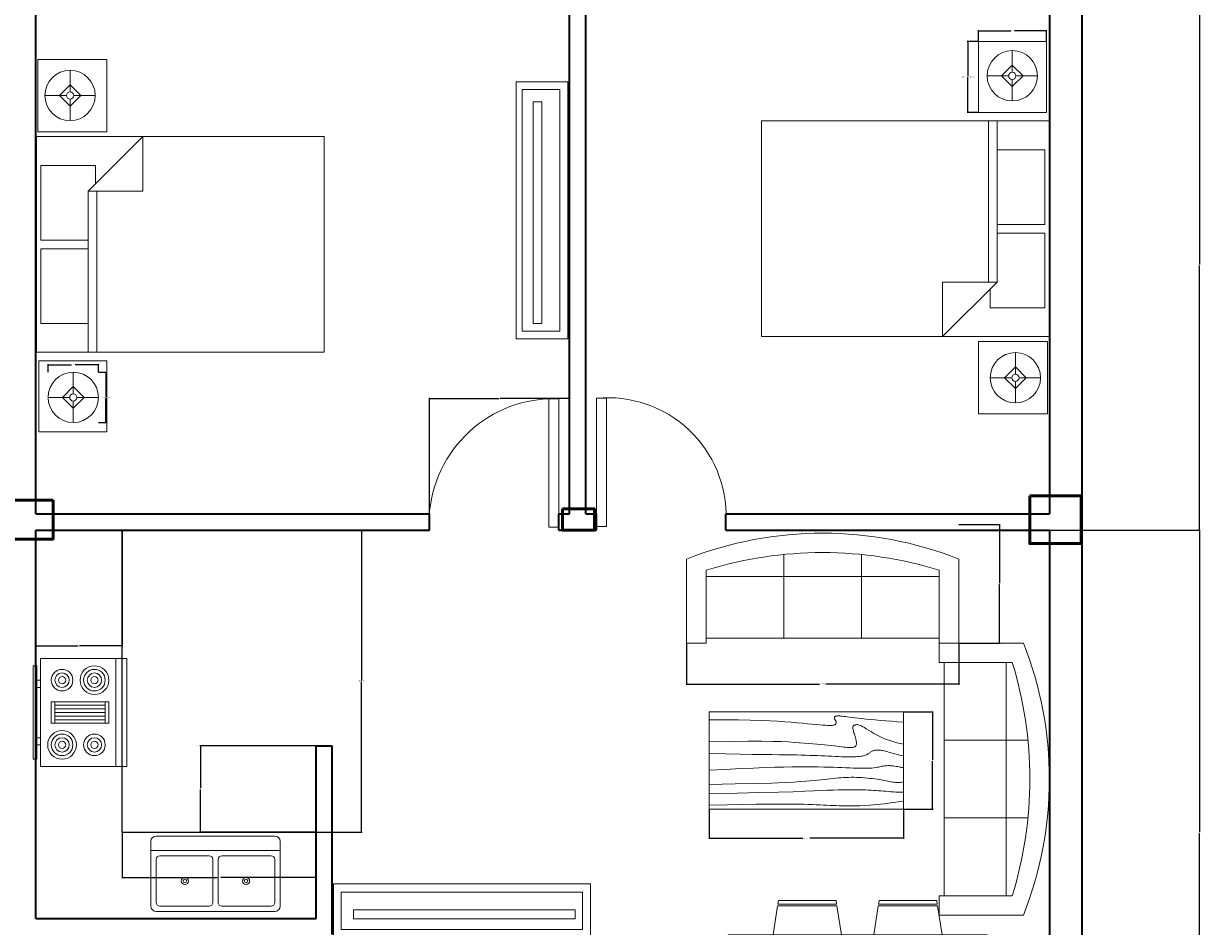
# Model space of a CAD drawing. Units: inches. Extents: x 50 to 2003, y -28 to 675.
# Tile 3 of 10: x 218 to 545, y 281 to 532. Entities that reach past the tile are written whole.
import ezdxf

# ---------------------------------------------------------------- set-up
doc = ezdxf.new("R2010")
doc.units = ezdxf.units.IN
for name, color, linetype, lineweight in [('A-ANNO-DIMS', 2, 'Continuous', 18), ('A-COLS', 1, 'Continuous', 50), ('A-DOOR', 4, 'Continuous', 18), ('A-EQPM', 8, 'Continuous', 18), ('A-FLOR-CASE', 32, 'Continuous', 25), ('A-FLOR-FIXT', 9, 'Continuous', 18), ('A-FURN', 8, 'Continuous', 18), ('A-FURN-LITE', 9, 'Continuous', 13), ('A-WALL', 7, 'Continuous', 35)]:
    doc.layers.add(name, color=color, linetype=linetype, lineweight=lineweight)
doc.styles.get("Standard").update_dxf_attribs({"font": 'arial.ttf'})
doc.dimstyles.get("Standard").update_dxf_attribs({"dimtxt": 0.18, "dimasz": 0.18, "dimexe": 0.18, "dimexo": 0.0625, "dimgap": 0.09, "dimtad": 0, "dimtih": 1, "dimtoh": 1, "dimdec": 4, "dimzin": 0, "dimdsep": 46, "dimtxsty": 'Standard', "dimcen": 0.09, "dimadec": 0, "dimazin": 0, "dimtfac": 1, "dimtdec": 4, "dimtofl": 0, "dimtmove": 0, "dimatfit": 3, "dimfxl": 1, "dimtolj": 1, "dimtzin": 0, "dimarcsym": 0})

# ---------------------------------------------------------------- blocks, each defined once
blk = doc.blocks.new('Sofa - Roundback 7 ft.')
for p, q in [((-12.00002, -32.4421), (-12.00003, -6.5971)), ((11.99997, -32.4421), (11.99998, -6.5971)), ((-36.000027, -34), (-36.000027, -11.4696)), ((-35.999844, -13.3819), (35.9998, -13.3819)), ((35.99998, -34), (35.99998, -11.4696)), ((-36.000027, -32.4421), (35.99998, -32.4421))]:
    blk.add_line(p, q)
for points in [[(-36.000027, -34), (-42.000027, -34), (-42.000027, -8)], [(41.99998, -8), (41.99998, -34), (35.99998, -34)]]:
    blk.add_lwpolyline(points)
for centre, radius, start, end in [((0, -114.25), 114.25, 68.43141, 111.5686), ((-0.00001, -127.1968), 121.1968, 72.72033, 107.2797)]:
    blk.add_arc(centre, radius, start, end)
blk = doc.blocks.new('Bed - Queen')
for p, q in [((0, -80.00003), (0, 0)), ((0, 0), (59.99999, 0)), ((59.99999, 0), (59.99999, -80.00003)), ((7.99999, -1.2), (28.79998, -1.2)), ((7.99999, -14.4), (7.99999, -1.2)), ((28.79998, -1.2), (28.79998, -14.4)), ((31.19999, -1.2), (51.99999, -1.2)), ((31.19999, -14.4), (31.19999, -1.2)), ((51.99999, -1.2), (51.99999, -16.4)), ((0, -14.4), (44.8, -14.4)), ((59.99999, -29.6), (44.8, -14.4)), ((44.8, -14.4), (44.8, -29.6)), ((44.8, -16.8), (0, -16.8)), ((51.99999, -16.4), (46.79936, -16.4)), ((44.8, -29.6), (59.99999, -29.6)), ((59.99999, -80.00003), (0, -80.00003))]:
    blk.add_line(p, q)
blk = doc.blocks.new('Lamp - Table')
for p, q in [((0, 7), (0, 1)), ((-1, 0), (-7, 0)), ((0, 3), (-3, 0)), ((-3, 0), (0, -3)), ((3, 0), (0, 3)), ((0, -3), (3, 0)), ((1, 0), (7, 0)), ((0, -1), (0, -7))]:
    blk.add_line(p, q)
for radius in [7, 1]:
    blk.add_circle((0, 0), radius)
blk = doc.blocks.new('Table - Rectangular Woodgrain 60 x 30 in.')
for p, q in [((0, 0), (0, -30)), ((60, 0), (0, 0)), ((60, -30), (60, 0)), ((0, -30), (60, -30))]:
    blk.add_line(p, q)
for points in [[(0, -2.4), (4.8155, -2.418), (9.0302, -2.4688), (12.709, -2.5477), (15.9167, -2.65), (18.7181, -2.7711), (21.1781, -2.9063), (23.3616, -3.0508), (25.3333, -3.2), (27.1477, -3.3495), (28.8172, -3.4958), (30.3437, -3.636), (31.7291, -3.7667), (32.9756, -3.8849), (34.0849, -3.9875), (35.059, -4.0714), (35.9, -4.1334), (36.6114, -4.1711), (37.2041, -4.1854), (37.6906, -4.1779), (38.0833, -4.15), (38.3948, -4.1034), (38.6375, -4.0396), (38.8239, -3.9602), (38.9666, -3.8667), (39.0764, -3.7608), (39.1573, -3.6448), (39.2116, -3.521), (39.2416, -3.3917), (39.2498, -3.2593), (39.2385, -3.1261), (39.21, -2.9944), (39.1666, -2.8667), (39.111, -2.7447), (39.0468, -2.6281), (38.978, -2.5163), (38.9083, -2.4083), (38.8418, -2.3035), (38.7823, -2.201), (38.7337, -2.1001), (38.7, -2), (38.6844, -1.9003), (38.6875, -1.8021), (38.7094, -1.707), (38.75, -1.6167), (38.8094, -1.5326), (38.8875, -1.4563), (38.9844, -1.3893), (39.1, -1.3333), (39.2351, -1.2896), (39.3937, -1.2583), (39.5804, -1.2396), (39.8, -1.2333), (40.057, -1.2396), (40.3562, -1.2583), (40.7023, -1.2896), (41.1, -1.3333), (41.5547, -1.3895), (42.0755, -1.4573), (42.6721, -1.5361), (43.3542, -1.625), (44.1316, -1.7233), (45.014, -1.8302), (46.0114, -1.9449), (47.1333, -2.0667), (48.3862, -2.1947), (49.7625, -2.3281), (51.2513, -2.4663), (52.8416, -2.6083), (54.5226, -2.7535), (56.2833, -2.9011), (58.1127, -3.0501), (60, -3.2)], [(0, -9.2), (6.5759, -9.0858), (11.9385, -9.0365), (16.2527, -9.0418), (19.6833, -9.0917), (22.3952, -9.1759), (24.5531, -9.2844), (26.322, -9.4069), (27.8666, -9.5333), (29.3241, -9.6553), (30.7203, -9.7719), (32.0532, -9.8837), (33.3208, -9.9917), (34.5213, -10.0965), (35.6526, -10.199), (36.7128, -10.2999), (37.7, -10.4), (38.6129, -10.4996), (39.4531, -10.5969), (40.223, -10.6895), (40.925, -10.775), (41.5613, -10.8512), (42.1344, -10.9156), (42.6465, -10.966), (43.1, -11), (43.4976, -11.0158), (43.8437, -11.0136), (44.143, -10.9942), (44.4, -10.9583), (44.6195, -10.9069), (44.8062, -10.8406), (44.9648, -10.7603), (45.1, -10.6667), (45.2155, -10.5598), (45.3114, -10.4365), (45.3871, -10.2929), (45.4416, -10.125), (45.4743, -9.929), (45.4844, -9.7011), (45.4709, -9.4371), (45.4333, -9.1333), (45.3716, -8.7883), (45.2896, -8.4104), (45.1919, -8.0107), (45.0833, -7.6), (44.9685, -7.1893), (44.8521, -6.7896), (44.7388, -6.4117), (44.6333, -6.0667), (44.54, -5.7628), (44.4614, -5.4979), (44.4001, -5.2675), (44.3583, -5.0667), (44.3384, -4.8909), (44.3427, -4.7354), (44.3736, -4.5956), (44.4333, -4.4667), (44.5236, -4.3453), (44.6427, -4.2333), (44.7884, -4.1339), (44.9583, -4.05), (45.1501, -3.9849), (45.3614, -3.9417), (45.59, -3.9234), (45.8333, -3.9333), (46.0915, -3.9749), (46.3734, -4.0531), (46.6906, -4.1736), (47.0542, -4.3417), (47.4756, -4.5629), (47.9661, -4.8427), (48.5372, -5.1866), (49.2, -5.6), (49.9676, -6.0844), (50.8594, -6.625), (51.8965, -7.2031), (53.1, -7.8), (54.491, -8.3969), (56.0906, -8.975), (57.9199, -9.5156), (60, -10)], [(0, -12.8), (5.1847, -12.9322), (9.6213, -13.0323), (13.3963, -13.1059), (16.5958, -13.1583), (19.3063, -13.1952), (21.614, -13.2219), (23.6054, -13.2439), (25.3666, -13.2667), (26.9728, -13.2947), (28.4531, -13.3281), (29.8256, -13.3663), (31.1083, -13.4083), (32.3191, -13.4535), (33.476, -13.501), (34.597, -13.5501), (35.7, -13.6), (36.7984, -13.6497), (37.8875, -13.6979), (38.9578, -13.743), (40, -13.7833), (41.0047, -13.8174), (41.9625, -13.8438), (42.864, -13.8607), (43.7, -13.8667), (44.4631, -13.8604), (45.1552, -13.8417), (45.7801, -13.8104), (46.3416, -13.7667), (46.8439, -13.7104), (47.2906, -13.6417), (47.6858, -13.5604), (48.0333, -13.4667), (48.3375, -13.3608), (48.6042, -13.2448), (48.8396, -13.121), (49.05, -12.9917), (49.2417, -12.8593), (49.4208, -12.7261), (49.5937, -12.5944), (49.7667, -12.4667), (49.9452, -12.3451), (50.1323, -12.2313), (50.3303, -12.1268), (50.5416, -12.0333), (50.7686, -11.9524), (51.0135, -11.8854), (51.2788, -11.8341), (51.5666, -11.8), (51.8785, -11.7843), (52.2116, -11.7865), (52.562, -11.8059), (52.926, -11.8417), (53.2998, -11.8931), (53.6795, -11.9594), (54.0614, -12.0397), (54.4416, -12.1333), (54.8223, -12.2401), (55.2293, -12.3625), (55.6942, -12.5037), (56.2489, -12.6667), (56.9251, -12.8547), (57.7545, -13.0708), (58.7689, -13.3182), (60, -13.6)], [(0, -18), (5.124, -17.7273), (9.6609, -17.5057), (13.6705, -17.3303), (17.2125, -17.1958), (20.3467, -17.0973), (23.1328, -17.0297), (25.6307, -16.9878), (27.9, -16.9667), (29.9928, -16.9617), (31.9302, -16.9703), (33.7254, -16.9907), (35.3917, -17.0208), (36.9423, -17.0588), (38.3906, -17.1026), (39.7499, -17.1503), (41.0333, -17.2), (42.2519, -17.2496), (43.4073, -17.2969), (44.4986, -17.3395), (45.525, -17.375), (46.4858, -17.4012), (47.3802, -17.4156), (48.2074, -17.416), (48.9667, -17.4), (49.6583, -17.3662), (50.2872, -17.3167), (50.8595, -17.2547), (51.3812, -17.1833), (51.8584, -17.1057), (52.2971, -17.025), (52.7034, -16.9443), (53.0833, -16.8667), (53.443, -16.7951), (53.789, -16.7313), (54.128, -16.6768), (54.4666, -16.6334), (54.8115, -16.6024), (55.1693, -16.5854), (55.5465, -16.5841), (55.95, -16.6), (56.3828, -16.6337), (56.8346, -16.6823), (57.2915, -16.7418), (57.7396, -16.8084), (58.165, -16.878), (58.5539, -16.9469), (58.8924, -17.0111), (59.1666, -17.0667), (59.3679, -17.1107), (59.5078, -17.1438), (59.6032, -17.1675), (59.6708, -17.1833), (59.7275, -17.193), (59.7901, -17.1979), (59.8753, -17.1998), (60, -17.2)], [(0, -22.4), (8.0098, -22.2501), (14.4094, -22.1011), (19.4168, -21.9535), (23.25, -21.8083), (26.1269, -21.6663), (28.2656, -21.5281), (29.884, -21.3947), (31.2, -21.2667), (32.3967, -21.1448), (33.5172, -21.0292), (34.5697, -20.9198), (35.5625, -20.8167), (36.5037, -20.7198), (37.4015, -20.6292), (38.2642, -20.5448), (39.1, -20.4667), (39.9164, -20.3951), (40.7187, -20.3313), (41.5117, -20.2768), (42.3, -20.2333), (43.0883, -20.2024), (43.8812, -20.1854), (44.6836, -20.1841), (45.5, -20.2), (46.3328, -20.234), (47.1747, -20.2844), (48.0163, -20.3488), (48.8479, -20.425), (49.66, -20.5106), (50.4429, -20.6031), (51.1872, -20.7004), (51.8833, -20.8), (52.5246, -20.8999), (53.1166, -20.9995), (53.6681, -21.0983), (54.1875, -21.1958), (54.6834, -21.2919), (55.1646, -21.3859), (55.6394, -21.4777), (56.1167, -21.5667), (56.6028, -21.6515), (57.0961, -21.7266), (57.5929, -21.7852), (58.0896, -21.8208), (58.5823, -21.8268), (59.0674, -21.7964), (59.5412, -21.723), (60, -21.6)], [(0, -25.2), (8.6355, -25.0504), (15.7026, -24.9031), (21.4049, -24.7606), (25.9458, -24.625), (29.529, -24.4988), (32.3578, -24.3844), (34.6359, -24.284), (36.5667, -24.2), (38.3213, -24.1341), (39.9417, -24.0854), (41.437, -24.0523), (42.8167, -24.0333), (44.0901, -24.0268), (45.2667, -24.0313), (46.3557, -24.0451), (47.3667, -24.0667), (48.309, -24.0947), (49.1928, -24.1287), (50.0284, -24.168), (50.826, -24.2125), (51.5959, -24.2617), (52.3483, -24.3151), (53.0935, -24.3725), (53.8417, -24.4334), (54.6009, -24.497), (55.3699, -24.561), (56.1454, -24.6226), (56.9239, -24.6792), (57.7021, -24.7279), (58.4764, -24.7662), (59.2435, -24.7911), (60, -24.8)], [(0, -28.8), (5.6867, -28.6681), (10.45, -28.5698), (14.407, -28.5012), (17.675, -28.4584), (20.3711, -28.4374), (22.6125, -28.4344), (24.5164, -28.4455), (26.2, -28.4667), (27.762, -28.4947), (29.2276, -28.5281), (30.6033, -28.5663), (31.8958, -28.6084), (33.1118, -28.6535), (34.2578, -28.7011), (35.3405, -28.7501), (36.3666, -28.8), (37.3443, -28.8497), (38.288, -28.8974), (39.2137, -28.9412), (40.1375, -28.9792), (41.0753, -29.0093), (42.0432, -29.0297), (43.0572, -29.0384), (44.1333, -29.0333), (45.2936, -29.0114), (46.5843, -28.9641), (48.0579, -28.8816), (49.7666, -28.7542), (51.7629, -28.5721), (54.0989, -28.3255), (56.8272, -28.0048), (60, -27.6)]]:
    blk.add_lwpolyline(points)
blk = doc.blocks.new('Dining Set - 36 x 72 in.')
for p, q in [((-22, 27.5), (-22.1562, 26.50042)), ((-5.8416, 26.5), (-22.1534, 26.5)), ((-22, 27.5), (-6, 27.5)), ((-5.8437, 26.49966), (-6, 27.5)), ((6, 27.5), (5.8438, 26.50042)), ((22.1584, 26.5), (5.8466, 26.5)), ((6, 27.5), (22, 27.5)), ((22.1563, 26.49966), (22, 27.5)), ((-22.2343, 26.00059), (-23.4847, 17.99762)), ((-22.2304, 26), (-5.7608, 26)), ((-4.5152, 17.99762), (-5.7655, 25.99926)), ((5.7657, 26.00059), (4.5153, 17.99762)), ((5.7696, 26), (22.2392, 26)), ((23.4848, 17.99762), (22.2345, 25.99926)), ((36, 18), (-36, 18)), ((-36, 18), (-36, -18)), ((36, -18), (36, 18)), ((-45.5, 8), (-44.5004, 8.15617)), ((-45.5, 8), (-45.5, -8)), ((-44.5, -8.15843), (-44.5, 8.15338)), ((-44.0006, 8.23428), (-35.9976, 9.48474)), ((-44, 8.23041), (-44, -8.23915)), ((44.0006, 8.23428), (35.9976, 9.48474)), ((44, 8.23041), (44, -8.23915)), ((44.5, -8.15843), (44.5, 8.15338)), ((45.5, 8), (44.5005, 8.15617)), ((45.5, 8), (45.5, -8)), ((-44.4997, -8.15631), (-45.5, -8)), ((-35.9976, -9.48476), (-43.9993, -8.2345)), ((35.9976, -9.48476), (43.9993, -8.2345)), ((44.4997, -8.15631), (45.5, -8)), ((-36, -18), (36, -18)), ((-22.2343, -26.0006), (-23.4847, -17.99762)), ((-4.5152, -17.99762), (-5.7655, -25.99928)), ((5.7657, -26.0006), (4.5153, -17.99762)), ((23.4848, -17.99762), (22.2345, -25.99928)), ((-22.2304, -26), (-5.7608, -26)), ((5.7696, -26), (22.2392, -26)), ((-22, -27.5), (-22.1562, -26.50044)), ((-5.8416, -26.5), (-22.1534, -26.5)), ((-22, -27.5), (-6, -27.5)), ((-5.8437, -26.49967), (-6, -27.5)), ((6, -27.5), (5.8438, -26.50044)), ((22.1584, -26.5), (5.8466, -26.5)), ((6, -27.5), (22, -27.5)), ((22.1563, -26.49967), (22, -27.5))]:
    blk.add_line(p, q)
for points in [[(-36, 15), (-31.1772, 14.97754), (-26.8079, 14.91406), (-22.8538, 14.81543), (-19.276, 14.6875), (-16.0362, 14.53613), (-13.0957, 14.36718), (-10.4159, 14.18652), (-7.9583, 14), (-5.6904, 13.81315), (-3.6035, 13.63021), (-1.6954, 13.45508), (0.0365, 13.29166), (1.5945, 13.14388), (2.9811, 13.01562), (4.1988, 12.9108), (5.25, 12.83333), (6.1393, 12.78613), (6.8802, 12.76823), (7.4883, 12.77767), (7.9792, 12.8125), (8.3685, 12.87077), (8.6719, 12.95052), (8.9049, 13.0498), (9.0833, 13.16666), (9.2205, 13.29899), (9.3216, 13.44401), (9.3895, 13.59879), (9.4271, 13.76041), (9.4373, 13.92594), (9.4232, 14.09245), (9.3875, 14.257), (9.3333, 14.41666), (9.2638, 14.56917), (9.1836, 14.71484), (9.0975, 14.85465), (9.0104, 14.98958), (8.9272, 15.1206), (8.8529, 15.2487), (8.7922, 15.37483), (8.75, 15.5), (8.7305, 15.62467), (8.7344, 15.74739), (8.7617, 15.86621), (8.8125, 15.97916), (8.8867, 16.08431), (8.9844, 16.17968), (9.1055, 16.26334), (9.25, 16.33333), (9.4189, 16.38802), (9.6172, 16.42708), (9.8506, 16.45052), (10.125, 16.45833), (10.4463, 16.45052), (10.8203, 16.42708), (11.2529, 16.38802), (11.75, 16.33333), (12.3184, 16.26318), (12.9694, 16.17838), (13.7151, 16.07991), (14.5677, 15.96875), (15.5395, 15.84586), (16.6426, 15.71224), (17.8893, 15.56884), (19.2917, 15.41666), (20.859, 15.25667), (22.5879, 15.08984), (24.4721, 14.91715), (26.5052, 14.73958), (28.6809, 14.5581), (30.9929, 14.3737), (33.4347, 14.18733), (36, 14)], [(-36, 10), (-28.9766, 10.14274), (-23.1725, 10.20442), (-18.4241, 10.19775), (-14.5677, 10.13541), (-11.4399, 10.03011), (-8.877, 9.89453), (-6.7154, 9.74137), (-4.7917, 9.58333), (-2.9698, 9.43082), (-1.2246, 9.28515), (0.4415, 9.14534), (2.026, 9.01041), (3.5266, 8.87939), (4.9408, 8.7513), (6.266, 8.62516), (7.5, 8.5), (8.6411, 8.37549), (9.6914, 8.2539), (10.6538, 8.13818), (11.5312, 8.03125), (12.3267, 7.93603), (13.043, 7.85547), (13.6831, 7.79248), (14.25, 7.75), (14.7471, 7.7303), (15.1797, 7.73307), (15.5537, 7.75732), (15.875, 7.80208), (16.1494, 7.86637), (16.3828, 7.94922), (16.5811, 8.04964), (16.75, 8.16666), (16.8944, 8.29915), (17.0143, 8.44531), (17.1089, 8.60319), (17.1771, 8.77083), (17.218, 8.94629), (17.2305, 9.1276), (17.2137, 9.31282), (17.1667, 9.5), (17.0895, 9.6875), (16.987, 9.875), (16.8649, 10.0625), (16.7292, 10.25), (16.5856, 10.4375), (16.4401, 10.625), (16.2985, 10.8125), (16.1667, 11), (16.05, 11.18733), (15.9518, 11.3737), (15.8752, 11.5581), (15.8229, 11.73958), (15.798, 11.91715), (15.8034, 12.08984), (15.842, 12.25667), (15.9167, 12.41666), (16.0295, 12.56836), (16.1784, 12.70833), (16.3605, 12.83268), (16.5729, 12.9375), (16.8127, 13.01888), (17.0768, 13.07291), (17.3625, 13.0957), (17.6667, 13.08333), (17.9894, 13.03312), (18.3418, 12.94726), (18.7382, 12.82918), (19.1927, 12.68229), (19.7195, 12.51001), (20.3327, 12.31575), (21.0465, 12.10294), (21.875, 11.875), (22.8357, 11.63354), (23.959, 11.37304), (25.2786, 11.08618), (26.8282, 10.76562), (28.6414, 10.40405), (30.752, 9.99414), (33.1936, 9.52856), (36, 9)], [(-36, 5.5), (-30.7157, 5.3348), (-26.069, 5.20963), (-21.9946, 5.11767), (-18.4271, 5.05208), (-15.3009, 5.00602), (-12.5508, 4.97265), (-10.1112, 4.94515), (-7.9167, 4.91666), (-5.909, 4.88167), (-4.0586, 4.83984), (-2.3429, 4.79215), (-0.7396, 4.73958), (0.7739, 4.6831), (2.22, 4.6237), (3.6213, 4.56233), (5, 4.5), (6.373, 4.43782), (7.7344, 4.3776), (9.0723, 4.32129), (10.375, 4.27083), (11.6309, 4.22819), (12.8281, 4.19531), (13.9551, 4.17415), (15, 4.16666), (15.954, 4.17448), (16.819, 4.19791), (17.6001, 4.23698), (18.3021, 4.29166), (18.9299, 4.36198), (19.4883, 4.44791), (19.9823, 4.54948), (20.4167, 4.66666), (20.7969, 4.79899), (21.1302, 4.94401), (21.4245, 5.09879), (21.6875, 5.26041), (21.9271, 5.42594), (22.1511, 5.59245), (22.3672, 5.757), (22.5834, 5.91666), (22.8065, 6.06868), (23.0404, 6.21093), (23.2879, 6.34147), (23.5521, 6.45833), (23.8358, 6.55957), (24.142, 6.64323), (24.4735, 6.70735), (24.8334, 6.75), (25.2235, 6.76969), (25.642, 6.76692), (26.0858, 6.74267), (26.5521, 6.69791), (27.0379, 6.63362), (27.5404, 6.55078), (28.0565, 6.45036), (28.5834, 6.33333), (29.1242, 6.19987), (29.7071, 6.04687), (30.3661, 5.87044), (31.1354, 5.66666), (32.0493, 5.43164), (33.142, 5.16146), (34.4475, 4.85221), (36, 4.5)], [(-36, -1), (-30.7915, -0.6591), (-26.0195, -0.38216), (-21.6519, -0.16284), (-17.6563, 0.00521), (-14.0005, 0.12833), (-10.6523, 0.21289), (-7.5796, 0.26522), (-4.75, 0.29166), (-2.134, 0.29793), (0.2878, 0.28711), (2.5317, 0.26163), (4.6146, 0.22396), (6.5529, 0.17651), (8.3633, 0.12174), (10.0623, 0.06209), (11.6667, 0), (13.1899, -0.06201), (14.6341, -0.1211), (15.9982, -0.17432), (17.2813, -0.21875), (18.4823, -0.25147), (19.6003, -0.26953), (20.6343, -0.27002), (21.5834, -0.25), (22.4481, -0.20768), (23.2357, -0.14584), (23.9549, -0.06836), (24.6146, 0.02083), (25.2235, 0.11784), (25.7904, 0.21875), (26.3241, 0.31966), (26.8334, 0.41666), (27.3265, 0.50618), (27.8099, 0.58593), (28.2894, 0.65397), (28.7709, 0.70833), (29.2601, 0.74707), (29.763, 0.76823), (30.2855, 0.76985), (30.8334, 0.75), (31.4088, 0.70784), (31.9994, 0.64713), (32.589, 0.57275), (33.1615, 0.48958), (33.7008, 0.4025), (34.1908, 0.3164), (34.6153, 0.23616), (34.9584, 0.16666), (35.2099, 0.11165), (35.3848, 0.07031), (35.504, 0.04069), (35.5886, 0.02083), (35.6594, 0.00879), (35.7377, 0.0026), (35.8442, 0.00032), (36, 0)], [(-36, -6.5), (-27.1843, -6.31267), (-20.084, -6.1263), (-14.469, -5.9419), (-10.1094, -5.76042), (-6.7752, -5.58285), (-4.2363, -5.41016), (-2.2629, -5.24333), (-0.625, -5.08334), (0.8708, -4.93099), (2.2715, -4.78646), (3.5872, -4.64974), (4.8281, -4.52084), (6.0046, -4.39974), (7.127, -4.28646), (8.2053, -4.18099), (9.25, -4.08334), (10.2705, -3.99382), (11.2734, -3.91407), (12.2647, -3.84603), (13.25, -3.79167), (14.2354, -3.75293), (15.2266, -3.73177), (16.2295, -3.73015), (17.25, -3.75), (18.2912, -3.79248), (19.3451, -3.85547), (20.4009, -3.93604), (21.4479, -4.03125), (22.4754, -4.13819), (23.4727, -4.25391), (24.4289, -4.37549), (25.3334, -4.5), (26.1785, -4.62492), (26.9694, -4.74935), (27.7145, -4.87281), (28.4219, -4.99479), (29.1, -5.11483), (29.7572, -5.23242), (30.4016, -5.34709), (31.0417, -5.45834), (31.6837, -5.56437), (32.3262, -5.65821), (32.9658, -5.73153), (33.599, -5.77604), (34.2224, -5.78345), (34.8327, -5.74545), (35.4264, -5.65373), (36, -5.5)], [(-36, -10), (-26.4022, -9.81299), (-18.4675, -9.62891), (-11.9839, -9.45069), (-6.7396, -9.28125), (-2.5226, -9.12354), (0.8789, -8.98047), (3.6769, -8.85498), (6.0833, -8.75), (8.2767, -8.66765), (10.3021, -8.60677), (12.1712, -8.56543), (13.8958, -8.54167), (15.4876, -8.53353), (16.9583, -8.53907), (18.3197, -8.55632), (19.5834, -8.58334), (20.7616, -8.61841), (21.8685, -8.66081), (22.9188, -8.71004), (23.9271, -8.76563), (24.9081, -8.82707), (25.8763, -8.89388), (26.8465, -8.96558), (27.8334, -9.04167), (28.8474, -9.12118), (29.8828, -9.20117), (30.93, -9.27824), (31.9792, -9.34896), (33.0205, -9.40991), (34.0443, -9.45768), (35.0407, -9.48885), (36, -9.5)], [(-36, -14.5), (-30.0881, -14.33513), (-25.0332, -14.21224), (-20.7312, -14.12647), (-17.0781, -14.07292), (-13.97, -14.04671), (-11.3027, -14.04297), (-8.9724, -14.05681), (-6.875, -14.08334), (-4.9224, -14.11833), (-3.0905, -14.16016), (-1.3709, -14.20785), (0.2448, -14.26042), (1.7647, -14.3169), (3.1973, -14.3763), (4.5507, -14.43767), (5.8333, -14.5), (7.0554, -14.5621), (8.235, -14.62175), (9.3922, -14.67652), (10.5469, -14.72396), (11.7192, -14.76164), (12.929, -14.78711), (14.1965, -14.79794), (15.5417, -14.79167), (16.9933, -14.76424), (18.6152, -14.70508), (20.4804, -14.60197), (22.6615, -14.44271), (25.2312, -14.21509), (28.2624, -13.9069), (31.8277, -13.50594), (36, -13)]]:
    blk.add_lwpolyline(points)
blk = doc.blocks.new('Range-Oven - 30 in top')
for p, q in [((0, -3), (30, -3)), ((12, -6), (18, -6)), ((13, -20), (13, -6)), ((14, -6), (14, -20)), ((15, -20), (15, -6)), ((16, -6), (16, -20)), ((17, -20), (17, -6)), ((18, -20), (12, -20)), ((6, -24), (6, -25)), ((8, -25), (8, -24)), ((22, -25), (22, -24)), ((24, -24), (24, -25))]:
    blk.add_line(p, q)
for points in [[(0, -24), (0, 0), (30, 0), (30, -24)], [(12, -21), (12, -5), (18, -5), (18, -21)], [(2, -26), (2, -25), (28, -25), (28, -26)]]:
    blk.add_lwpolyline(points, close=True)
for centre, radius in [((6, -9), 4), ((6, -9), 3), ((24, -9), 3), ((6, -9), 2), ((6, -9), 1), ((24, -9), 2), ((24, -9), 1), ((6, -18), 3), ((6, -18), 2), ((24, -18), 4), ((24, -18), 3), ((24, -18), 2), ((6, -18), 1), ((24, -18), 1)]:
    blk.add_circle(centre, radius)
blk = doc.blocks.new('Sink-double - 36 in top')
for p, q in [((-18, -4), (18, -4)), ((-0.75, -18.5), (-0.75, -6.5)), ((0.75, -6.5), (0.75, -18.5))]:
    blk.add_line(p, q)
for points in [[(-16.5, 0), (16.5, 0)], [(-18, -19.5), (-18, -1.5)], [(18, -1.5), (18, -19.5)], [(-16.5, -18.5), (-16.5, -6.5)], [(-15.5, -5.5), (-1.75, -5.5)], [(1.75, -5.5), (15.5, -5.5)], [(16.5, -6.5), (16.5, -18.5)], [(-1.75, -19.5), (-15.5, -19.5)], [(15.5, -19.5), (1.75, -19.5)], [(16.5, -21), (-16.5, -21)]]:
    blk.add_lwpolyline(points)
for centre, radius in [((-8.5, -12.5), 1), ((-8.5, -12.5), 0.5), ((8.5, -12.5), 1), ((8.5, -12.5), 0.5)]:
    blk.add_circle(centre, radius)
for centre, radius, start, end in [((-16.5, -1.5), 1.5, 90, 180), ((16.5, -1.5), 1.5, 0, 90), ((-15.5, -6.5), 1, 90, 180), ((-1.75, -6.5), 1, 0, 90), ((1.75, -6.5), 1, 90, 180), ((15.5, -6.5), 1, 0, 90), ((-16.5, -19.5), 1.5, 180, 270), ((-15.5, -18.5), 1, 180, 270), ((-1.75, -18.5), 1, 270, 0), ((1.75, -18.5), 1, 180, 270), ((15.5, -18.5), 1, 270, 0), ((16.5, -19.5), 1.5, 270, 0)]:
    blk.add_arc(centre, radius, start, end)
blk = doc.blocks.new('KITCHEN-COUNTER-L')
for q in [(0, 84), (54, 0)]:
    blk.add_line((0, 0), q)
blk = doc.blocks.new('MEDIA-CONSOLE')
for points in [[(0, 0), (71.49, 0), (71.49, 14.4), (0, 14.4)], [(2.13, 1.7), (69.3, 1.7), (69.3, 12.15), (2.13, 12.15)], [(5.56, 4.74), (67.2, 4.74), (67.2, 7.16), (5.56, 7.16)]]:
    blk.add_lwpolyline(points, close=True)
blk = doc.blocks.new('DOOR-LEAF-36')
blk.add_lwpolyline([(35.71, 2.81), (35.71, 0), (0, 0), (0, 2.81)], close=True)
blk = doc.blocks.new('NIGHTSTAND-COMPACT')
blk.add_lwpolyline([(0, 19.73), (0, 0), (18.92, 0), (18.92, 19.73)], close=True)
blk = doc.blocks.new('NIGHTSTAND-STANDARD')
blk.add_lwpolyline([(0, 0), (0, 20.13), (19.19, 20.13), (19.19, 0)], close=True)
blk = doc.blocks.new('*D19')
at = {"layer": 'A-ANNO-DIMS', "color": 0, "lineweight": -2, "transparency": 16777216}
for p, q in [((238.47, 435.23), (240.69, 435.23)), ((240.51, 435.05), (240.51, 428.41)), ((240.51, 421.41), (240.51, 428.05)), ((238.47, 421.23), (240.69, 421.23))]:
    blk.add_line(p, q, dxfattribs=at)
at = {"layer": 'A-ANNO-DIMS', "color": 0, "transparency": 16777216}
for points in [[(240.48, 435.05), (240.54, 435.05), (240.51, 435.23)], [(240.48, 421.41), (240.54, 421.41), (240.51, 421.23)]]:
    blk.add_solid(points, dxfattribs=at)
at = {"layer": 'Defpoints', "color": 0, "transparency": 16777216}
for p in [(238.41, 435.23), (240.51, 435.23), (238.41, 421.23)]:
    blk.add_point(p, dxfattribs=at)
at = {"layer": 'A-ANNO-DIMS', "color": 0, "transparency": 16777216, "insert": (240.51, 428.23), "char_height": 0.18, "attachment_point": 5}
blk.add_mtext('\\A1;TABLE LAMP 14 TYP.', dxfattribs=at)
blk = doc.blocks.new('*D20')
at = {"layer": 'A-ANNO-DIMS', "color": 0, "lineweight": -2, "transparency": 16777216}
for p, q in [((224.41, 435.3), (224.41, 437.51)), ((224.59, 437.33), (230.89, 437.33)), ((238.23, 437.33), (231.93, 437.33)), ((238.41, 435.3), (238.41, 437.51))]:
    blk.add_line(p, q, dxfattribs=at)
at = {"layer": 'A-ANNO-DIMS', "color": 0, "transparency": 16777216}
for points in [[(224.59, 437.36), (224.59, 437.3), (224.41, 437.33)], [(238.23, 437.36), (238.23, 437.3), (238.41, 437.33)]]:
    blk.add_solid(points, dxfattribs=at)
at = {"layer": 'Defpoints', "color": 0, "transparency": 16777216}
for p in [(224.41, 437.33), (224.41, 435.23), (238.41, 435.23)]:
    blk.add_point(p, dxfattribs=at)
at = {"layer": 'A-ANNO-DIMS', "color": 0, "transparency": 16777216, "insert": (231.41, 437.33), "char_height": 0.18, "attachment_point": 5}
blk.add_mtext('\\A1;14 TYP.', dxfattribs=at)
blk = doc.blocks.new('*D25')
at = {"layer": 'A-ANNO-DIMS', "color": 0, "lineweight": -2, "transparency": 16777216}
for p, q in [((483.19, 527.26), (480.11, 527.26)), ((480.29, 527.08), (480.29, 517.58)), ((480.29, 507.71), (480.29, 517.21)), ((483.19, 507.53), (480.11, 507.53))]:
    blk.add_line(p, q, dxfattribs=at)
at = {"layer": 'A-ANNO-DIMS', "color": 0, "transparency": 16777216}
for points in [[(480.26, 527.08), (480.32, 527.08), (480.29, 527.26)], [(480.26, 507.71), (480.32, 507.71), (480.29, 507.53)]]:
    blk.add_solid(points, dxfattribs=at)
at = {"layer": 'Defpoints', "color": 0, "transparency": 16777216}
for p in [(483.25, 527.26), (480.29, 507.53), (483.25, 507.53)]:
    blk.add_point(p, dxfattribs=at)
at = {"layer": 'A-ANNO-DIMS', "color": 0, "transparency": 16777216, "insert": (480.29, 517.39), "char_height": 0.18, "attachment_point": 5}
blk.add_mtext('\\A1;COMPACT NIGHTSTAND 20 TYP.', dxfattribs=at)
blk = doc.blocks.new('*D26')
at = {"layer": 'A-ANNO-DIMS', "color": 0, "lineweight": -2, "transparency": 16777216}
for p, q in [((483.25, 527.32), (483.25, 530.4)), ((502.17, 527.32), (502.17, 530.4)), ((483.43, 530.22), (492.19, 530.22)), ((501.99, 530.22), (493.23, 530.22))]:
    blk.add_line(p, q, dxfattribs=at)
at = {"layer": 'A-ANNO-DIMS', "color": 0, "transparency": 16777216}
for points in [[(483.43, 530.25), (483.43, 530.19), (483.25, 530.22)], [(501.99, 530.25), (501.99, 530.19), (502.17, 530.22)]]:
    blk.add_solid(points, dxfattribs=at)
at = {"layer": 'Defpoints', "color": 0, "transparency": 16777216}
for p in [(483.25, 530.22), (483.25, 527.26), (502.17, 527.26)]:
    blk.add_point(p, dxfattribs=at)
at = {"layer": 'A-ANNO-DIMS', "color": 0, "transparency": 16777216, "insert": (492.71, 530.22), "char_height": 0.18, "attachment_point": 5}
blk.add_mtext('\\A1;19 TYP.', dxfattribs=at)
blk = doc.blocks.new('*D35')
at = {"layer": 'A-ANNO-DIMS', "color": 0, "lineweight": -2, "transparency": 16777216}
for p, q in [((402.03, 359.78), (402.03, 348.31)), ((477.73, 359.78), (477.73, 348.31)), ((402.21, 348.49), (438.97, 348.49)), ((477.55, 348.49), (440.78, 348.49))]:
    blk.add_line(p, q, dxfattribs=at)
at = {"layer": 'A-ANNO-DIMS', "color": 0, "transparency": 16777216}
for points in [[(402.21, 348.52), (402.21, 348.46), (402.03, 348.49)], [(477.55, 348.52), (477.55, 348.46), (477.73, 348.49)]]:
    blk.add_solid(points, dxfattribs=at)
at = {"layer": 'Defpoints', "color": 0, "transparency": 16777216}
for p in [(402.03, 359.84), (477.73, 359.84), (477.73, 348.49)]:
    blk.add_point(p, dxfattribs=at)
at = {"layer": 'A-ANNO-DIMS', "color": 0, "transparency": 16777216, "insert": (439.88, 348.49), "char_height": 0.18, "attachment_point": 5}
blk.add_mtext('\\A1;SOFA 76 TYP.', dxfattribs=at)
blk = doc.blocks.new('*D36')
at = {"layer": 'A-ANNO-DIMS', "color": 0, "lineweight": -2, "transparency": 16777216}
for p, q in [((477.79, 392.89), (489.26, 392.89)), ((489.08, 392.71), (489.08, 376.55)), ((489.08, 360.02), (489.08, 376.18)), ((477.79, 359.84), (489.26, 359.84))]:
    blk.add_line(p, q, dxfattribs=at)
at = {"layer": 'A-ANNO-DIMS', "color": 0, "transparency": 16777216}
for points in [[(489.05, 392.71), (489.11, 392.71), (489.08, 392.89)], [(489.05, 360.02), (489.11, 360.02), (489.08, 359.84)]]:
    blk.add_solid(points, dxfattribs=at)
at = {"layer": 'Defpoints', "color": 0, "transparency": 16777216}
for p in [(477.73, 392.89), (489.08, 392.89), (477.73, 359.84)]:
    blk.add_point(p, dxfattribs=at)
at = {"layer": 'A-ANNO-DIMS', "color": 0, "transparency": 16777216, "insert": (489.08, 376.37), "char_height": 0.18, "attachment_point": 5}
blk.add_mtext('\\A1;33 TYP.', dxfattribs=at)
blk = doc.blocks.new('*D45')
at = {"layer": 'A-ANNO-DIMS', "color": 0, "lineweight": -2, "transparency": 16777216}
for p, q in [((408.27, 313.66), (408.27, 305.43)), ((462.34, 313.66), (462.34, 305.43)), ((408.45, 305.61), (434.33, 305.61)), ((462.16, 305.61), (436.27, 305.61))]:
    blk.add_line(p, q, dxfattribs=at)
at = {"layer": 'A-ANNO-DIMS', "color": 0, "transparency": 16777216}
for points in [[(408.45, 305.64), (408.45, 305.58), (408.27, 305.61)], [(462.16, 305.64), (462.16, 305.58), (462.34, 305.61)]]:
    blk.add_solid(points, dxfattribs=at)
at = {"layer": 'Defpoints', "color": 0, "transparency": 16777216}
for p in [(408.27, 313.72), (462.34, 313.72), (462.34, 305.61)]:
    blk.add_point(p, dxfattribs=at)
at = {"layer": 'A-ANNO-DIMS', "color": 0, "transparency": 16777216, "insert": (435.3, 305.61), "char_height": 0.18, "attachment_point": 5}
blk.add_mtext('\\A1;LOW TABLE 54', dxfattribs=at)
blk = doc.blocks.new('*D46')
at = {"layer": 'A-ANNO-DIMS', "color": 0, "lineweight": -2, "transparency": 16777216}
for p, q in [((462.4, 340.76), (470.63, 340.76)), ((470.45, 340.58), (470.45, 327.42)), ((470.45, 313.9), (470.45, 327.06)), ((462.4, 313.72), (470.63, 313.72))]:
    blk.add_line(p, q, dxfattribs=at)
at = {"layer": 'A-ANNO-DIMS', "color": 0, "transparency": 16777216}
for points in [[(470.42, 340.58), (470.48, 340.58), (470.45, 340.76)], [(470.42, 313.9), (470.48, 313.9), (470.45, 313.72)]]:
    blk.add_solid(points, dxfattribs=at)
at = {"layer": 'Defpoints', "color": 0, "transparency": 16777216}
for p in [(462.34, 340.76), (470.45, 340.76), (462.34, 313.72)]:
    blk.add_point(p, dxfattribs=at)
at = {"layer": 'A-ANNO-DIMS', "color": 0, "transparency": 16777216, "insert": (470.45, 327.24), "char_height": 0.18, "attachment_point": 5}
blk.add_mtext('\\A1;27', dxfattribs=at)
blk = doc.blocks.new('*D49')
at = {"layer": 'A-ANNO-DIMS', "color": 0, "lineweight": -2, "transparency": 16777216}
for p, q in [((299.03, 391.32), (311.75, 391.32)), ((311.57, 391.14), (311.57, 349.51)), ((311.57, 307.5), (311.57, 349.14)), ((299.03, 307.32), (311.75, 307.32))]:
    blk.add_line(p, q, dxfattribs=at)
at = {"layer": 'A-ANNO-DIMS', "color": 0, "transparency": 16777216}
for points in [[(311.54, 391.14), (311.6, 391.14), (311.57, 391.32)], [(311.54, 307.5), (311.6, 307.5), (311.57, 307.32)]]:
    blk.add_solid(points, dxfattribs=at)
at = {"layer": 'Defpoints', "color": 0, "transparency": 16777216}
for p in [(298.97, 391.32), (311.57, 391.32), (298.97, 307.32)]:
    blk.add_point(p, dxfattribs=at)
at = {"layer": 'A-ANNO-DIMS', "color": 0, "transparency": 16777216, "insert": (311.57, 349.32), "char_height": 0.18, "attachment_point": 5}
blk.add_mtext('\\A1;COUNTER 84 TYP.', dxfattribs=at)
blk = doc.blocks.new('*D50')
at = {"layer": 'A-ANNO-DIMS', "color": 0, "lineweight": -2, "transparency": 16777216}
for p, q in [((244.97, 307.26), (244.97, 294.54)), ((298.97, 307.26), (298.97, 294.54)), ((245.15, 294.72), (271.44, 294.72)), ((298.79, 294.72), (272.5, 294.72))]:
    blk.add_line(p, q, dxfattribs=at)
at = {"layer": 'A-ANNO-DIMS', "color": 0, "transparency": 16777216}
for points in [[(245.15, 294.75), (245.15, 294.69), (244.97, 294.72)], [(298.79, 294.75), (298.79, 294.69), (298.97, 294.72)]]:
    blk.add_solid(points, dxfattribs=at)
at = {"layer": 'Defpoints', "color": 0, "transparency": 16777216}
for p in [(244.97, 307.32), (298.97, 307.32), (298.97, 294.72)]:
    blk.add_point(p, dxfattribs=at)
at = {"layer": 'A-ANNO-DIMS', "color": 0, "transparency": 16777216, "insert": (271.97, 294.72), "char_height": 0.18, "attachment_point": 5}
blk.add_mtext('\\A1;54 TYP.', dxfattribs=at)
blk = doc.blocks.new('*D61')
at = {"layer": 'A-ANNO-DIMS', "color": 0, "lineweight": -2, "transparency": 16777216}
for p, q in [((503.03, 391.32), (544.84, 391.32)), ((544.66, 391.14), (544.66, 307.26)), ((544.66, 223), (544.66, 306.89)), ((503.03, 222.82), (544.84, 222.82))]:
    blk.add_line(p, q, dxfattribs=at)
at = {"layer": 'A-ANNO-DIMS', "color": 0, "transparency": 16777216}
for points in [[(544.63, 391.14), (544.69, 391.14), (544.66, 391.32)], [(544.63, 223), (544.69, 223), (544.66, 222.82)]]:
    blk.add_solid(points, dxfattribs=at)
at = {"layer": 'Defpoints', "color": 0, "transparency": 16777216}
for p in [(502.97, 391.32), (544.66, 391.32), (502.97, 222.82)]:
    blk.add_point(p, dxfattribs=at)
at = {"layer": 'A-ANNO-DIMS', "color": 0, "transparency": 16777216, "insert": (544.66, 307.07), "char_height": 0.18, "attachment_point": 5}
blk.add_mtext('\\A1;168.5', dxfattribs=at)
blk = doc.blocks.new('*D62')
at = {"layer": 'A-ANNO-DIMS', "color": 0, "lineweight": -2, "transparency": 16777216}
for p, q in [((503.03, 538.82), (544.84, 538.82)), ((544.66, 538.64), (544.66, 465.26)), ((544.66, 391.5), (544.66, 464.89)), ((503.03, 391.32), (544.84, 391.32))]:
    blk.add_line(p, q, dxfattribs=at)
at = {"layer": 'A-ANNO-DIMS', "color": 0, "transparency": 16777216}
for points in [[(544.63, 538.64), (544.69, 538.64), (544.66, 538.82)], [(544.63, 391.5), (544.69, 391.5), (544.66, 391.32)]]:
    blk.add_solid(points, dxfattribs=at)
at = {"layer": 'Defpoints', "color": 0, "transparency": 16777216}
for p in [(502.97, 538.82), (544.66, 538.82), (502.97, 391.32)]:
    blk.add_point(p, dxfattribs=at)
at = {"layer": 'A-ANNO-DIMS', "color": 0, "transparency": 16777216, "insert": (544.66, 465.07), "char_height": 0.18, "attachment_point": 5}
blk.add_mtext('\\A1;147.5', dxfattribs=at)
blk = doc.blocks.new('*D70')
at = {"layer": 'A-ANNO-DIMS', "color": 0, "lineweight": -2, "transparency": 16777216}
for p, q in [((330.47, 395.89), (330.47, 428.15)), ((330.65, 427.97), (349.75, 427.97)), ((369.29, 427.97), (350.19, 427.97)), ((369.47, 395.89), (369.47, 428.15))]:
    blk.add_line(p, q, dxfattribs=at)
at = {"layer": 'A-ANNO-DIMS', "color": 0, "transparency": 16777216}
for points in [[(330.65, 428), (330.65, 427.94), (330.47, 427.97)], [(369.29, 428), (369.29, 427.94), (369.47, 427.97)]]:
    blk.add_solid(points, dxfattribs=at)
at = {"layer": 'Defpoints', "color": 0, "transparency": 16777216}
for p in [(369.47, 427.97), (330.47, 395.82), (369.47, 395.82)]:
    blk.add_point(p, dxfattribs=at)
at = {"layer": 'A-ANNO-DIMS', "color": 0, "transparency": 16777216, "insert": (349.97, 427.97), "char_height": 0.18, "attachment_point": 5}
blk.add_mtext('\\A1;39', dxfattribs=at)
blk = doc.blocks.new('*D72')
at = {"layer": 'A-ANNO-DIMS', "color": 0, "lineweight": -2, "transparency": 16777216}
for p, q in [((298.91, 331.32), (266.64, 331.32)), ((266.82, 331.14), (266.82, 319.5)), ((266.82, 307.5), (266.82, 319.14)), ((298.91, 307.32), (266.64, 307.32))]:
    blk.add_line(p, q, dxfattribs=at)
at = {"layer": 'A-ANNO-DIMS', "color": 0, "transparency": 16777216}
for points in [[(266.79, 331.14), (266.85, 331.14), (266.82, 331.32)], [(266.79, 307.5), (266.85, 307.5), (266.82, 307.32)]]:
    blk.add_solid(points, dxfattribs=at)
at = {"layer": 'Defpoints', "color": 0, "transparency": 16777216}
for p in [(266.82, 331.32), (298.97, 331.32), (298.97, 307.32)]:
    blk.add_point(p, dxfattribs=at)
at = {"layer": 'A-ANNO-DIMS', "color": 0, "transparency": 16777216, "insert": (266.82, 319.32), "char_height": 0.18, "attachment_point": 5}
blk.add_mtext('\\A1;24', dxfattribs=at)
blk = doc.blocks.new('*D73')
at = {"layer": 'A-ANNO-DIMS', "color": 0, "lineweight": -2, "transparency": 16777216}
for p, q in [((220.97, 391.26), (220.97, 358.99)), ((244.97, 391.26), (244.97, 358.99)), ((221.15, 359.17), (232.75, 359.17)), ((244.79, 359.17), (233.19, 359.17))]:
    blk.add_line(p, q, dxfattribs=at)
at = {"layer": 'A-ANNO-DIMS', "color": 0, "transparency": 16777216}
for points in [[(221.15, 359.2), (221.15, 359.14), (220.97, 359.17)], [(244.79, 359.2), (244.79, 359.14), (244.97, 359.17)]]:
    blk.add_solid(points, dxfattribs=at)
at = {"layer": 'Defpoints', "color": 0, "transparency": 16777216}
for p in [(220.97, 391.32), (244.97, 391.32), (220.97, 359.17)]:
    blk.add_point(p, dxfattribs=at)
at = {"layer": 'A-ANNO-DIMS', "color": 0, "transparency": 16777216, "insert": (232.97, 359.17), "char_height": 0.18, "attachment_point": 5}
blk.add_mtext('\\A1;24', dxfattribs=at)

msp = doc.modelspace()

# ---------------------------------------------------------------- linework, layer by layer
at = {"layer": 'A-COLS'}
for points in [[(225.7742, 399.6502), (211.9886, 399.6502), (211.9886, 388.811), (225.7742, 388.811)], [(497.4538, 400.8924), (511.7851, 400.8924), (511.7851, 387.5858), (497.4538, 387.5858)], [(367.4719, 397.2412), (376.3768, 397.2412), (376.3768, 391.3411), (367.4719, 391.3411)]]:
    msp.add_lwpolyline(points, close=True, dxfattribs=at)
at = {"layer": 'A-DOOR'}
for centre, radius, start, end in [((365.0682, 393.168), 34.701, 87.741102, 177.331859), ((380.104, 395.2495), 32.9079, 358.326228, 95.325929)]:
    msp.add_arc(centre, radius, start, end, dxfattribs=at)
at = {"layer": 'A-WALL'}
for p, q in [((511.9711, 642.3232), (511.9711, 17.3232)), ((220.9711, 395.8232), (220.9711, 538.8232)), ((369.4711, 395.8232), (369.4711, 538.8232)), ((373.9711, 395.8232), (373.9711, 538.8232)), ((502.9711, 538.8232), (502.9711, 395.8232)), ((220.9711, 395.8232), (330.4711, 395.8232)), ((330.4711, 391.3232), (330.4711, 395.8232)), ((366.4711, 391.3232), (366.4711, 395.8232)), ((366.4711, 395.8232), (369.4711, 395.8232)), ((373.9711, 395.8232), (376.9711, 395.8232)), ((376.9711, 391.3232), (376.9711, 395.8232)), ((412.9711, 391.3232), (412.9711, 395.8232)), ((412.9711, 395.8232), (502.9711, 395.8232)), ((220.9711, 391.3232), (330.4711, 391.3232)), ((220.9711, 283.3232), (220.9711, 391.3232)), ((366.4711, 391.3232), (376.9711, 391.3232)), ((412.9711, 391.3232), (502.9711, 391.3232)), ((502.9711, 391.3232), (502.9711, 227.3232)), ((298.9711, 283.3232), (298.9711, 331.3232)), ((298.9711, 331.3232), (303.4711, 331.3232)), ((303.4711, 278.8232), (303.4711, 331.3232)), ((220.9711, 283.3232), (298.9711, 283.3232))]:
    msp.add_line(p, q, dxfattribs=at)

# ---------------------------------------------------------------- block references
at = {"layer": 'A-DOOR'}
for p, rotation in [((363.6685, 427.8886), 270.0000000000001), ((376.9686, 428.0599), 269.9999999999999)]:
    msp.add_blockref('DOOR-LEAF-36', p, dxfattribs=dict(at, rotation=rotation))
at = {"layer": 'A-EQPM', "rotation": 270}
msp.add_blockref('Range-Oven - 30 in top', (246.2964, 355.5912), dxfattribs=at)
at = {"layer": 'A-FLOR-CASE'}
msp.add_blockref('KITCHEN-COUNTER-L', (244.9711, 307.3232), dxfattribs=at)
at = {"layer": 'A-FLOR-FIXT'}
msp.add_blockref('Sink-double - 36 in top', (270.9672, 306.2313), dxfattribs=at)
at = {"layer": 'A-FURN'}
for name, p, rotation in [('NIGHTSTAND-COMPACT', (502.1701, 527.2611), 180), ('MEDIA-CONSOLE', (354.6211, 516.0001), 270.0000000000001), ('Bed - Queen', (502.8303, 505.1447), 270), ('Bed - Queen', (221.2007, 440.7953), 90), ('NIGHTSTAND-STANDARD', (502.4366, 443.791), 180)]:
    msp.add_blockref(name, p, dxfattribs=dict(at, rotation=rotation))
for name, p in [('NIGHTSTAND-STANDARD', (221.5944, 502.1489)), ('NIGHTSTAND-COMPACT', (221.8609, 418.6788)), ('MEDIA-CONSOLE', (303.7949, 278.4981)), ('Dining Set - 36 x 72 in.', (449.5836, 260.7888))]:
    msp.add_blockref(name, p, dxfattribs=at)
at = {"layer": 'A-FURN', "xscale": 0.901192412465213, "yscale": 0.901192412465213, "zscale": 0.901192412465213}
for name, p in [('Sofa - Roundback 7 ft.', (439.8767, 390.484)), ('Table - Rectangular Woodgrain 60 x 30 in.', (408.2665, 340.7583))]:
    msp.add_blockref(name, p, dxfattribs=at)
at = {"layer": 'A-FURN', "xscale": 0.901192412465213, "yscale": 0.901192412465213, "zscale": 0.901192412465213, "rotation": 270}
msp.add_blockref('Sofa - Roundback 7 ft.', (502.9296, 322.0752), dxfattribs=at)
at = {"layer": 'A-FURN-LITE'}
for p, rotation in [((492.6219, 517.7068), 270), ((230.5361, 512.231), 90), ((493.4949, 433.709), 270), ((231.4091, 428.2332), 90)]:
    msp.add_blockref('Lamp - Table', p, dxfattribs=dict(at, rotation=rotation))

# ---------------------------------------------------------------- dimensions: what is measured, and where the dimension line sits
at = {"layer": 'A-ANNO-DIMS'}
for base, p1, p2, angle, override, picture, middle in [((544.6551, 538.8232), (502.9711, 391.3232), (502.9711, 538.8232), 90, {"dimdec": 1, "dimlfac": 1, "dimrnd": 0, "dimzin": 0, "dimdsep": 46, "dimlunit": 2}, '*D62', (544.6551, 465.0732)), ((220.9711, 359.1732), (244.9711, 391.3232), (220.9711, 391.3232), 180, {"dimdec": 0, "dimlfac": 1, "dimrnd": 0, "dimzin": 0, "dimdsep": 46, "dimlunit": 2}, '*D73', (232.9711, 359.1732)), ((544.6551, 391.3232), (502.9711, 222.8232), (502.9711, 391.3232), 90, {"dimdec": 1, "dimlfac": 1, "dimrnd": 0, "dimzin": 0, "dimdsep": 46, "dimlunit": 2}, '*D61', (544.6551, 307.0732)), ((470.4488, 340.7583), (462.338, 313.7225), (462.338, 340.7583), 90, {"dimdec": 0, "dimlfac": 1, "dimrnd": 0, "dimzin": 0, "dimdsep": 46, "dimlunit": 2}, '*D46', (470.4488, 327.2404)), ((266.8211, 331.3232), (298.9711, 307.3232), (298.9711, 331.3232), 90, {"dimdec": 0, "dimlfac": 1, "dimrnd": 0, "dimzin": 0, "dimdsep": 46, "dimlunit": 2}, '*D72', (266.8211, 319.3232))]:
    dim = msp.add_linear_dim(base=base, p1=p1, p2=p2, angle=angle, dimstyle='Standard', override=override, dxfattribs=at)
    dim.commit()
    dim.dimension.update_dxf_attribs({"geometry": picture, "text_midpoint": middle})
for base, p1, p2, angle, text, picture, middle in [((483.2478, 530.2212), (502.1701, 527.2611), (483.2478, 527.2611), 180, '<> TYP.', '*D26', (492.709, 530.2212)), ((480.2877, 507.527), (483.2478, 527.2611), (483.2478, 507.527), 270, 'COMPACT NIGHTSTAND <> TYP.', '*D25', (480.2877, 517.394)), ((224.4091, 437.3332), (238.4091, 435.2332), (224.4091, 435.2332), 180, '<> TYP.', '*D20', (231.4091, 437.3332)), ((240.5091, 435.2332), (238.4091, 421.2332), (238.4091, 435.2332), 90, 'TABLE LAMP <> TYP.', '*D19', (240.5091, 428.2332)), ((489.0818, 392.8872), (477.7268, 359.8435), (477.7268, 392.8872), 90, '<> TYP.', '*D36', (489.0818, 376.3653)), ((311.5711, 391.3232), (298.9711, 307.3232), (298.9711, 391.3232), 90, 'COUNTER <> TYP.', '*D49', (311.5711, 349.3232))]:
    dim = msp.add_linear_dim(base=base, p1=p1, p2=p2, angle=angle, text=text, dimstyle='Standard', override={"dimdec": 0, "dimlfac": 1, "dimrnd": 0, "dimzin": 0, "dimdsep": 46, "dimlunit": 2}, dxfattribs=at)
    dim.commit()
    dim.dimension.update_dxf_attribs({"geometry": picture, "text_midpoint": middle})
dim = msp.add_linear_dim(base=(369.4711, 427.9732), p1=(330.4711, 395.8232), p2=(369.4711, 395.8232), dimstyle='Standard', override={"dimdec": 0, "dimlfac": 1, "dimrnd": 0, "dimzin": 0, "dimdsep": 46, "dimlunit": 2}, dxfattribs=at)
dim.commit()
dim.dimension.update_dxf_attribs({"geometry": '*D70', "text_midpoint": (349.9711, 427.9732)})
for base, p1, p2, text, picture, middle in [((477.7268, 348.4884), (402.0266, 359.8435), (477.7268, 359.8435), 'SOFA <> TYP.', '*D35', (439.8767, 348.4884)), ((462.338, 305.6118), (408.2665, 313.7225), (462.338, 313.7225), 'LOW TABLE <>', '*D45', (435.3023, 305.6118)), ((298.9711, 294.7232), (244.9711, 307.3232), (298.9711, 307.3232), '<> TYP.', '*D50', (271.9711, 294.7232))]:
    dim = msp.add_linear_dim(base=base, p1=p1, p2=p2, text=text, dimstyle='Standard', override={"dimdec": 0, "dimlfac": 1, "dimrnd": 0, "dimzin": 0, "dimdsep": 46, "dimlunit": 2}, dxfattribs=at)
    dim.commit()
    dim.dimension.update_dxf_attribs({"geometry": picture, "text_midpoint": middle})

doc.saveas('drawing.dxf')
